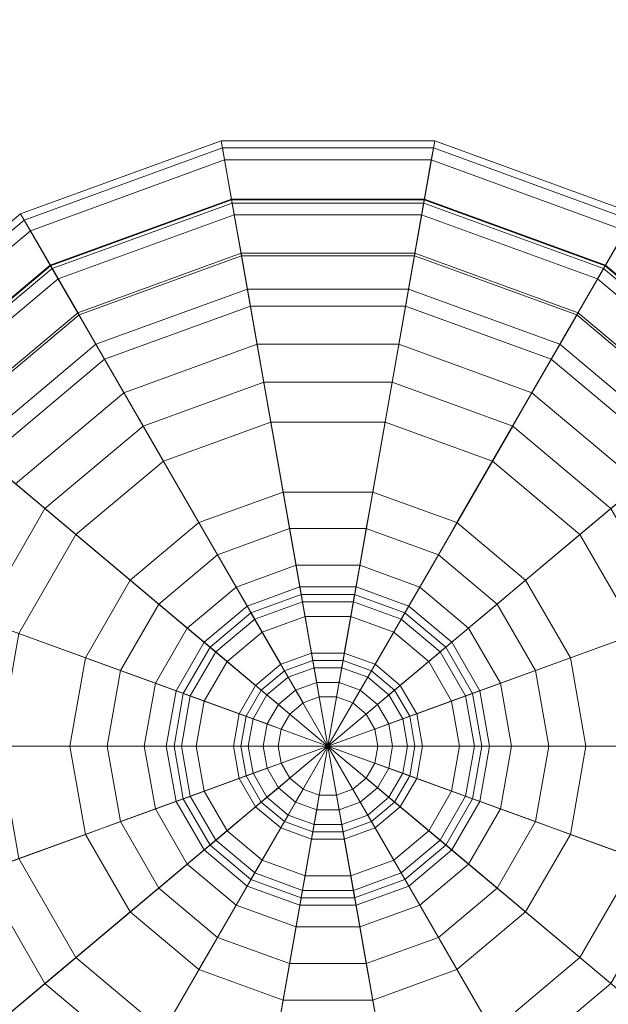
# Model space of a CAD drawing. Units: inches. Extents: x 375 to 1122, y 27 to 1069.
# Tile 110 of 155: x 732.383 to 733.68, y 872.701 to 874.871. Entities that reach past the tile are written whole.
import ezdxf

# ---------------------------------------------------------------- set-up
doc = ezdxf.new("R2010")
doc.units = ezdxf.units.IN
doc.layers.add('A-ANNO-DIMS', color=2, linetype='Continuous', lineweight=18)
doc.layers.add('Furniture', color=30, linetype='Continuous', lineweight=18)
doc.styles.get("Standard").update_dxf_attribs({"font": 'arial.ttf'})
doc.dimstyles.new('ISO-25', dxfattribs={"dimtxt": 12, "dimasz": 2.5, "dimexe": 1.5, "dimexo": 1.5, "dimtad": 1, "dimdec": 1, "dimlunit": 3, "dimtxsty": 'Standard', "dimblk": 'ARCHTICK', "dimcen": 2.5, "dimadec": 0, "dimazin": 0, "dimtfac": 1, "dimtdec": 1, "dimtmove": 0, "dimatfit": 3, "dimfxl": 1.5, "dimfxlon": 1, "dimarcsym": 0})

# ---------------------------------------------------------------- blocks, each defined once
blk = doc.blocks.new('A$C403C54AD')
for points in [[(1.626464, 1.23678, -0.04658), (1.626464, 1.202917, -0.043501), (1.626464, 1.202917, -0.043501), (1.614883, 1.234737, -0.04658)], [(1.638046, 1.234737, -0.04658), (1.626464, 1.202917, -0.043501), (1.626464, 1.202917, -0.043501), (1.626464, 1.23678, -0.04658)], [(1.614883, 1.234737, -0.04658), (1.626464, 1.202917, -0.043501), (1.626464, 1.202917, -0.043501), (1.604698, 1.228857, -0.04658)], [(1.64823, 1.228857, -0.04658), (1.626464, 1.202917, -0.043501), (1.626464, 1.202917, -0.043501), (1.638046, 1.234737, -0.04658)], [(1.626464, 1.217132, -0.040074), (1.626464, 1.233514, -0.043349), (1.616, 1.231669, -0.043349), (1.621603, 1.216274, -0.040074)], [(1.631326, 1.216274, -0.040074), (1.636929, 1.231669, -0.043349), (1.626464, 1.233514, -0.043349), (1.626464, 1.217132, -0.040074)], [(1.621603, 1.216274, -0.040074), (1.616, 1.231669, -0.043349), (1.606797, 1.226356, -0.043349), (1.617327, 1.213806, -0.040074)], [(1.635601, 1.213806, -0.040074), (1.646131, 1.226356, -0.043349), (1.636929, 1.231669, -0.043349), (1.631326, 1.216274, -0.040074)], [(1.604698, 1.228857, -0.04658), (1.626464, 1.202917, -0.043501), (1.626464, 1.202917, -0.043501), (1.597139, 1.219849, -0.04658)], [(1.606797, 1.226356, -0.043349), (1.604698, 1.228857, -0.04658), (1.597139, 1.219849, -0.04658), (1.599967, 1.218216, -0.043349)], [(1.65579, 1.219849, -0.04658), (1.626464, 1.202917, -0.043501), (1.626464, 1.202917, -0.043501), (1.64823, 1.228857, -0.04658)], [(1.606823, 1.226325, 0.116404), (1.604954, 1.228552, 0.10318), (1.597484, 1.219649, 0.10318), (1.600002, 1.218195, 0.116404)], [(1.605388, 1.228035, 0.074938), (1.608836, 1.223925, 0.056929), (1.602714, 1.216629, 0.056929), (1.598069, 1.219312, 0.074938)], [(1.617327, 1.213806, -0.040074), (1.606797, 1.226356, -0.043349), (1.599967, 1.218216, -0.043349), (1.614154, 1.210025, -0.040074)], [(1.610035, 1.222497, 0.12581), (1.606823, 1.226325, 0.116404), (1.600002, 1.218195, 0.116404), (1.604329, 1.215697, 0.12581)], [(1.606937, 1.226189, 0.102963), (1.608743, 1.224037, 0.115599), (1.602589, 1.216702, 0.115599), (1.600155, 1.218107, 0.102963)], [(1.60736, 1.225685, 0.075423), (1.606937, 1.226189, 0.102963), (1.600155, 1.218107, 0.102963), (1.600725, 1.217778, 0.075423)], [(1.620264, 1.219951, 0.048884), (1.618046, 1.226046, 0.058276), (1.610643, 1.221772, 0.058276), (1.614812, 1.216804, 0.048884)], [(1.638116, 1.216804, 0.048884), (1.642285, 1.221772, 0.058276), (1.634882, 1.226046, 0.058276), (1.632664, 1.219951, 0.048884)], [(1.638774, 1.210025, -0.040074), (1.652961, 1.218216, -0.043349), (1.646131, 1.226356, -0.043349), (1.635601, 1.213806, -0.040074)], [(1.610643, 1.221772, 0.058276), (1.60736, 1.225685, 0.075423), (1.600725, 1.217778, 0.075423), (1.605149, 1.215224, 0.058276)], [(1.608743, 1.224037, 0.115599), (1.612014, 1.220139, 0.12581), (1.606995, 1.214158, 0.12581), (1.602589, 1.216702, 0.115599)], [(1.608836, 1.223925, 0.056929), (1.613379, 1.218512, 0.046697), (1.608834, 1.213096, 0.046697), (1.602714, 1.216629, 0.056929)], [(1.650214, 1.216629, 0.056929), (1.644094, 1.213096, 0.046697), (1.63955, 1.218512, 0.046697), (1.644092, 1.223925, 0.056929)], [(1.626464, 1.223275, 0.046697), (1.626464, 1.213036, 0.03933), (1.623003, 1.212426, 0.03933), (1.619501, 1.222047, 0.046697)], [(1.633427, 1.222047, 0.046697), (1.629925, 1.212426, 0.03933), (1.626464, 1.213036, 0.03933), (1.626464, 1.223275, 0.046697)], [(1.612014, 1.220139, 0.12581), (1.610035, 1.222497, 0.12581), (1.604329, 1.215697, 0.12581), (1.606995, 1.214158, 0.12581)], [(1.614812, 1.216804, 0.048884), (1.610643, 1.221772, 0.058276), (1.605149, 1.215224, 0.058276), (1.610766, 1.211981, 0.048884)], [(1.619501, 1.222047, 0.046697), (1.623003, 1.212426, 0.03933), (1.61996, 1.210669, 0.03933), (1.613379, 1.218512, 0.046697)], [(1.63955, 1.218512, 0.046697), (1.632968, 1.210669, 0.03933), (1.629925, 1.212426, 0.03933), (1.633427, 1.222047, 0.046697)], [(1.642163, 1.211981, 0.048884), (1.64778, 1.215224, 0.058276), (1.642285, 1.221772, 0.058276), (1.638116, 1.216804, 0.048884)], [(1.626464, 1.211822, 0.042248), (1.626464, 1.221045, 0.048884), (1.620264, 1.219951, 0.048884), (1.623419, 1.211285, 0.042248)], [(1.62951, 1.211285, 0.042248), (1.632664, 1.219951, 0.048884), (1.626464, 1.221045, 0.048884), (1.626464, 1.211822, 0.042248)], [(1.623419, 1.211285, 0.042248), (1.620264, 1.219951, 0.048884), (1.614812, 1.216804, 0.048884), (1.620741, 1.209738, 0.042248)], [(1.632188, 1.209738, 0.042248), (1.638116, 1.216804, 0.048884), (1.632664, 1.219951, 0.048884), (1.62951, 1.211285, 0.042248)], [(1.597139, 1.219849, -0.04658), (1.626464, 1.202917, -0.043501), (1.626464, 1.202917, -0.043501), (1.593116, 1.208798, -0.04658)], [(1.599967, 1.218216, -0.043349), (1.597139, 1.219849, -0.04658), (1.593116, 1.208798, -0.04658), (1.596333, 1.20823, -0.043349)], [(1.600002, 1.218195, 0.116404), (1.597484, 1.219649, 0.10318), (1.593509, 1.208728, 0.10318), (1.596372, 1.208223, 0.116404)], [(1.597484, 1.219649, 0.10318), (1.598069, 1.219312, 0.074938), (1.594174, 1.208611, 0.074938), (1.593509, 1.208728, 0.10318)], [(1.659812, 1.208798, -0.04658), (1.626464, 1.202917, -0.043501), (1.626464, 1.202917, -0.043501), (1.65579, 1.219849, -0.04658)], [(1.598069, 1.219312, 0.074938), (1.602714, 1.216629, 0.056929), (1.599457, 1.20768, 0.056929), (1.594174, 1.208611, 0.074938)], [(1.613379, 1.218512, 0.046697), (1.61996, 1.210669, 0.03933), (1.617701, 1.207977, 0.03933), (1.608834, 1.213096, 0.046697)], [(1.644094, 1.213096, 0.046697), (1.635227, 1.207977, 0.03933), (1.632968, 1.210669, 0.03933), (1.63955, 1.218512, 0.046697)], [(1.614154, 1.210025, -0.040074), (1.599967, 1.218216, -0.043349), (1.596333, 1.20823, -0.043349), (1.612466, 1.205386, -0.040074)], [(1.604329, 1.215697, 0.12581), (1.600002, 1.218195, 0.116404), (1.596372, 1.208223, 0.116404), (1.601293, 1.207356, 0.12581)], [(1.600155, 1.218107, 0.102963), (1.602589, 1.216702, 0.115599), (1.599314, 1.207705, 0.115599), (1.596547, 1.208193, 0.102963)], [(1.600725, 1.217778, 0.075423), (1.600155, 1.218107, 0.102963), (1.596547, 1.208193, 0.102963), (1.597195, 1.208078, 0.075423)], [(1.605149, 1.215224, 0.058276), (1.600725, 1.217778, 0.075423), (1.597195, 1.208078, 0.075423), (1.602225, 1.207191, 0.058276)], [(1.640462, 1.205386, -0.040074), (1.656596, 1.20823, -0.043349), (1.652961, 1.218216, -0.043349), (1.638774, 1.210025, -0.040074)], [(1.602589, 1.216702, 0.115599), (1.606995, 1.214158, 0.12581), (1.604324, 1.206821, 0.12581), (1.599314, 1.207705, 0.115599)], [(1.620741, 1.209738, 0.042248), (1.614812, 1.216804, 0.048884), (1.610766, 1.211981, 0.048884), (1.618753, 1.207369, 0.042248)], [(1.626464, 1.215084, -0.037209), (1.626464, 1.217132, -0.040074), (1.621603, 1.216274, -0.040074), (1.622303, 1.21435, -0.037209)], [(1.630625, 1.21435, -0.037209), (1.631326, 1.216274, -0.040074), (1.626464, 1.217132, -0.040074), (1.626464, 1.215084, -0.037209)], [(1.634175, 1.207369, 0.042248), (1.642163, 1.211981, 0.048884), (1.638116, 1.216804, 0.048884), (1.632188, 1.209738, 0.042248)], [(1.602714, 1.216629, 0.056929), (1.608834, 1.213096, 0.046697), (1.606416, 1.206452, 0.046697), (1.599457, 1.20768, 0.056929)], [(1.622303, 1.21435, -0.037209), (1.621603, 1.216274, -0.040074), (1.617327, 1.213806, -0.040074), (1.618644, 1.212238, -0.037209)], [(1.634285, 1.212238, -0.037209), (1.635601, 1.213806, -0.040074), (1.631326, 1.216274, -0.040074), (1.630625, 1.21435, -0.037209)], [(1.606995, 1.214158, 0.12581), (1.604329, 1.215697, 0.12581), (1.601293, 1.207356, 0.12581), (1.604324, 1.206821, 0.12581)], [(1.610766, 1.211981, 0.048884), (1.605149, 1.215224, 0.058276), (1.602225, 1.207191, 0.058276), (1.608612, 1.206065, 0.048884)], [(1.626464, 1.210988, -0.035163), (1.626464, 1.215084, -0.037209), (1.622303, 1.21435, -0.037209), (1.623704, 1.210502, -0.035163)], [(1.629225, 1.210502, -0.035163), (1.630625, 1.21435, -0.037209), (1.626464, 1.215084, -0.037209), (1.626464, 1.210988, -0.035163)], [(1.623704, 1.210502, -0.035163), (1.622303, 1.21435, -0.037209), (1.618644, 1.212238, -0.037209), (1.621276, 1.2091, -0.035163)], [(1.631652, 1.2091, -0.035163), (1.634285, 1.212238, -0.037209), (1.630625, 1.21435, -0.037209), (1.629225, 1.210502, -0.035163)], [(1.618644, 1.212238, -0.037209), (1.617327, 1.213806, -0.040074), (1.614154, 1.210025, -0.040074), (1.615928, 1.209001, -0.037209)], [(1.637001, 1.209001, -0.037209), (1.638774, 1.210025, -0.040074), (1.635601, 1.213806, -0.040074), (1.634285, 1.212238, -0.037209)], [(1.608834, 1.213096, 0.046697), (1.617701, 1.207977, 0.03933), (1.616499, 1.204675, 0.03933), (1.606416, 1.206452, 0.046697)], [(1.626464, 1.213036, 0.03933), (1.626464, 1.208122, 0.038511), (1.624684, 1.207808, 0.038511), (1.623003, 1.212426, 0.03933)], [(1.629925, 1.212426, 0.03933), (1.628244, 1.207808, 0.038511), (1.626464, 1.208122, 0.038511), (1.626464, 1.213036, 0.03933)], [(1.646512, 1.206452, 0.046697), (1.636429, 1.204675, 0.03933), (1.635227, 1.207977, 0.03933), (1.644094, 1.213096, 0.046697)], [(1.623003, 1.212426, 0.03933), (1.624684, 1.207808, 0.038511), (1.623119, 1.206904, 0.038511), (1.61996, 1.210669, 0.03933)], [(1.632968, 1.210669, 0.03933), (1.629809, 1.206904, 0.038511), (1.628244, 1.207808, 0.038511), (1.629925, 1.212426, 0.03933)], [(1.618753, 1.207369, 0.042248), (1.610766, 1.211981, 0.048884), (1.608612, 1.206065, 0.048884), (1.617695, 1.204464, 0.042248)], [(1.621276, 1.2091, -0.035163), (1.618644, 1.212238, -0.037209), (1.615928, 1.209001, -0.037209), (1.619474, 1.206953, -0.035163)], [(1.626464, 1.202917, 0.040765), (1.626464, 1.211822, 0.042248), (1.623419, 1.211285, 0.042248), (1.626464, 1.202917, 0.040765)], [(1.626464, 1.202917, 0.040765), (1.62951, 1.211285, 0.042248), (1.626464, 1.211822, 0.042248), (1.626464, 1.202917, 0.040765)], [(1.633454, 1.206953, -0.035163), (1.637001, 1.209001, -0.037209), (1.634285, 1.212238, -0.037209), (1.631652, 1.2091, -0.035163)], [(1.635233, 1.204464, 0.042248), (1.644316, 1.206065, 0.048884), (1.642163, 1.211981, 0.048884), (1.634175, 1.207369, 0.042248)], [(1.626464, 1.202917, 0.040765), (1.623419, 1.211285, 0.042248), (1.620741, 1.209738, 0.042248), (1.626464, 1.202917, 0.040765)], [(1.626464, 1.211398, 0.035646), (1.626464, 1.207302, 0.033599), (1.624964, 1.207038, 0.033599), (1.623564, 1.210887, 0.035646)], [(1.626464, 1.210169, 0.037692), (1.626464, 1.211398, 0.035646), (1.623564, 1.210887, 0.035646), (1.623984, 1.209732, 0.037692)], [(1.629365, 1.210887, 0.035646), (1.627964, 1.207038, 0.033599), (1.626464, 1.207302, 0.033599), (1.626464, 1.211398, 0.035646)], [(1.628944, 1.209732, 0.037692), (1.629365, 1.210887, 0.035646), (1.626464, 1.211398, 0.035646), (1.626464, 1.210169, 0.037692)], [(1.626464, 1.202917, 0.040765), (1.632188, 1.209738, 0.042248), (1.62951, 1.211285, 0.042248), (1.626464, 1.202917, 0.040765)], [(1.623564, 1.210887, 0.035646), (1.624964, 1.207038, 0.033599), (1.623646, 1.206277, 0.033599), (1.621013, 1.209414, 0.035646)], [(1.623984, 1.209732, 0.037692), (1.623564, 1.210887, 0.035646), (1.621013, 1.209414, 0.035646), (1.621803, 1.208473, 0.037692)], [(1.626464, 1.207712, -0.029842), (1.626464, 1.210988, -0.035163), (1.623704, 1.210502, -0.035163), (1.624824, 1.207423, -0.029842)], [(1.628104, 1.207423, -0.029842), (1.629225, 1.210502, -0.035163), (1.626464, 1.210988, -0.035163), (1.626464, 1.207712, -0.029842)], [(1.631915, 1.209414, 0.035646), (1.629283, 1.206277, 0.033599), (1.627964, 1.207038, 0.033599), (1.629365, 1.210887, 0.035646)], [(1.631126, 1.208473, 0.037692), (1.631915, 1.209414, 0.035646), (1.629365, 1.210887, 0.035646), (1.628944, 1.209732, 0.037692)], [(1.61996, 1.210669, 0.03933), (1.623119, 1.206904, 0.038511), (1.621957, 1.205519, 0.038511), (1.617701, 1.207977, 0.03933)], [(1.624824, 1.207423, -0.029842), (1.623704, 1.210502, -0.035163), (1.621276, 1.2091, -0.035163), (1.623382, 1.20659, -0.029842)], [(1.629546, 1.20659, -0.029842), (1.631652, 1.2091, -0.035163), (1.629225, 1.210502, -0.035163), (1.628104, 1.207423, -0.029842)], [(1.635227, 1.207977, 0.03933), (1.630971, 1.205519, 0.038511), (1.629809, 1.206904, 0.038511), (1.632968, 1.210669, 0.03933)], [(1.615928, 1.209001, -0.037209), (1.614154, 1.210025, -0.040074), (1.612466, 1.205386, -0.040074), (1.614482, 1.20503, -0.037209)], [(1.626464, 1.202917, 0.040765), (1.620741, 1.209738, 0.042248), (1.618753, 1.207369, 0.042248), (1.626464, 1.202917, 0.040765)], [(1.624684, 1.207808, 0.038511), (1.623984, 1.209732, 0.037692), (1.621803, 1.208473, 0.037692), (1.623119, 1.206904, 0.038511)], [(1.626464, 1.208122, 0.038511), (1.626464, 1.210169, 0.037692), (1.623984, 1.209732, 0.037692), (1.624684, 1.207808, 0.038511)], [(1.628244, 1.207808, 0.038511), (1.628944, 1.209732, 0.037692), (1.626464, 1.210169, 0.037692), (1.626464, 1.208122, 0.038511)], [(1.626464, 1.202917, 0.040765), (1.634175, 1.207369, 0.042248), (1.632188, 1.209738, 0.042248), (1.626464, 1.202917, 0.040765)], [(1.629809, 1.206904, 0.038511), (1.631126, 1.208473, 0.037692), (1.628944, 1.209732, 0.037692), (1.628244, 1.207808, 0.038511)], [(1.638446, 1.20503, -0.037209), (1.640462, 1.205386, -0.040074), (1.638774, 1.210025, -0.040074), (1.637001, 1.209001, -0.037209)], [(1.621013, 1.209414, 0.035646), (1.623646, 1.206277, 0.033599), (1.622667, 1.20511, 0.033599), (1.61912, 1.207158, 0.035646)], [(1.621803, 1.208473, 0.037692), (1.621013, 1.209414, 0.035646), (1.61912, 1.207158, 0.035646), (1.620184, 1.206543, 0.037692)], [(1.623382, 1.20659, -0.029842), (1.621276, 1.2091, -0.035163), (1.619474, 1.206953, -0.035163), (1.622312, 1.205315, -0.029842)], [(1.633809, 1.207158, 0.035646), (1.630262, 1.20511, 0.033599), (1.629283, 1.206277, 0.033599), (1.631915, 1.209414, 0.035646)], [(1.630616, 1.205315, -0.029842), (1.633454, 1.206953, -0.035163), (1.631652, 1.2091, -0.035163), (1.629546, 1.20659, -0.029842)], [(1.632744, 1.206543, 0.037692), (1.633809, 1.207158, 0.035646), (1.631915, 1.209414, 0.035646), (1.631126, 1.208473, 0.037692)], [(1.593116, 1.208798, -0.04658), (1.626464, 1.202917, -0.043501), (1.626464, 1.202917, -0.043501), (1.593116, 1.197037, -0.04658)], [(1.596333, 1.20823, -0.043349), (1.593116, 1.208798, -0.04658), (1.593116, 1.197037, -0.04658), (1.596333, 1.197604, -0.043349)], [(1.596372, 1.208223, 0.116404), (1.593509, 1.208728, 0.10318), (1.593509, 1.197107, 0.10318), (1.596372, 1.197611, 0.116404)], [(1.593509, 1.208728, 0.10318), (1.594174, 1.208611, 0.074938), (1.594174, 1.197224, 0.074938), (1.593509, 1.197107, 0.10318)], [(1.594174, 1.208611, 0.074938), (1.599457, 1.20768, 0.056929), (1.599457, 1.198155, 0.056929), (1.594174, 1.197224, 0.074938)], [(1.619474, 1.206953, -0.035163), (1.615928, 1.209001, -0.037209), (1.614482, 1.20503, -0.037209), (1.618516, 1.204319, -0.035163)], [(1.659812, 1.197037, -0.04658), (1.626464, 1.202917, -0.043501), (1.626464, 1.202917, -0.043501), (1.659812, 1.208798, -0.04658)], [(1.634413, 1.204319, -0.035163), (1.638446, 1.20503, -0.037209), (1.637001, 1.209001, -0.037209), (1.633454, 1.206953, -0.035163)], [(1.612466, 1.205386, -0.040074), (1.596333, 1.20823, -0.043349), (1.596333, 1.197604, -0.043349), (1.612466, 1.200449, -0.040074)], [(1.601293, 1.207356, 0.12581), (1.596372, 1.208223, 0.116404), (1.596372, 1.197611, 0.116404), (1.601293, 1.198479, 0.12581)], [(1.596547, 1.208193, 0.102963), (1.599314, 1.207705, 0.115599), (1.599314, 1.19813, 0.115599), (1.596547, 1.197642, 0.102963)], [(1.597195, 1.208078, 0.075423), (1.596547, 1.208193, 0.102963), (1.596547, 1.197642, 0.102963), (1.597195, 1.197756, 0.075423)], [(1.602225, 1.207191, 0.058276), (1.597195, 1.208078, 0.075423), (1.597195, 1.197756, 0.075423), (1.602225, 1.198643, 0.058276)], [(1.623119, 1.206904, 0.038511), (1.621803, 1.208473, 0.037692), (1.620184, 1.206543, 0.037692), (1.621957, 1.205519, 0.038511)], [(1.630971, 1.205519, 0.038511), (1.632744, 1.206543, 0.037692), (1.631126, 1.208473, 0.037692), (1.629809, 1.206904, 0.038511)], [(1.640462, 1.200449, -0.040074), (1.656596, 1.197604, -0.043349), (1.656596, 1.20823, -0.043349), (1.640462, 1.205386, -0.040074)], [(1.599314, 1.207705, 0.115599), (1.604324, 1.206821, 0.12581), (1.604324, 1.199014, 0.12581), (1.599314, 1.19813, 0.115599)], [(1.599457, 1.20768, 0.056929), (1.606416, 1.206452, 0.046697), (1.606416, 1.199382, 0.046697), (1.599457, 1.198155, 0.056929)], [(1.617701, 1.207977, 0.03933), (1.621957, 1.205519, 0.038511), (1.621339, 1.203821, 0.038511), (1.616499, 1.204675, 0.03933)], [(1.626464, 1.206483, -0.021247), (1.626464, 1.207712, -0.029842), (1.624824, 1.207423, -0.029842), (1.625245, 1.206268, -0.021247)], [(1.627684, 1.206268, -0.021247), (1.628104, 1.207423, -0.029842), (1.626464, 1.207712, -0.029842), (1.626464, 1.206483, -0.021247)], [(1.636429, 1.204675, 0.03933), (1.631589, 1.203821, 0.038511), (1.630971, 1.205519, 0.038511), (1.635227, 1.207977, 0.03933)], [(1.604324, 1.206821, 0.12581), (1.601293, 1.207356, 0.12581), (1.601293, 1.198479, 0.12581), (1.604324, 1.199014, 0.12581)], [(1.608612, 1.206065, 0.048884), (1.602225, 1.207191, 0.058276), (1.602225, 1.198643, 0.058276), (1.608612, 1.19977, 0.048884)], [(1.626464, 1.202917, 0.040765), (1.618753, 1.207369, 0.042248), (1.617695, 1.204464, 0.042248), (1.626464, 1.202917, 0.040765)], [(1.61912, 1.207158, 0.035646), (1.622667, 1.20511, 0.033599), (1.622146, 1.203679, 0.033599), (1.618112, 1.20439, 0.035646)], [(1.620184, 1.206543, 0.037692), (1.61912, 1.207158, 0.035646), (1.618112, 1.20439, 0.035646), (1.619322, 1.204177, 0.037692)], [(1.622312, 1.205315, -0.029842), (1.619474, 1.206953, -0.035163), (1.618516, 1.204319, -0.035163), (1.621742, 1.20375, -0.029842)], [(1.625245, 1.206268, -0.021247), (1.624824, 1.207423, -0.029842), (1.623382, 1.20659, -0.029842), (1.624172, 1.205649, -0.021247)], [(1.624964, 1.207038, 0.033599), (1.625525, 1.205499, 0.027051), (1.624699, 1.205022, 0.027051), (1.623646, 1.206277, 0.033599)], [(1.626464, 1.207302, 0.033599), (1.626464, 1.205664, 0.027051), (1.625525, 1.205499, 0.027051), (1.624964, 1.207038, 0.033599)], [(1.626464, 1.202917, 0.040765), (1.635233, 1.204464, 0.042248), (1.634175, 1.207369, 0.042248), (1.626464, 1.202917, 0.040765)], [(1.627964, 1.207038, 0.033599), (1.627404, 1.205499, 0.027051), (1.626464, 1.205664, 0.027051), (1.626464, 1.207302, 0.033599)], [(1.629283, 1.206277, 0.033599), (1.62823, 1.205022, 0.027051), (1.627404, 1.205499, 0.027051), (1.627964, 1.207038, 0.033599)], [(1.628756, 1.205649, -0.021247), (1.629546, 1.20659, -0.029842), (1.628104, 1.207423, -0.029842), (1.627684, 1.206268, -0.021247)], [(1.634816, 1.20439, 0.035646), (1.630783, 1.203679, 0.033599), (1.630262, 1.20511, 0.033599), (1.633809, 1.207158, 0.035646)], [(1.631186, 1.20375, -0.029842), (1.634413, 1.204319, -0.035163), (1.633454, 1.206953, -0.035163), (1.630616, 1.205315, -0.029842)], [(1.633606, 1.204177, 0.037692), (1.634816, 1.20439, 0.035646), (1.633809, 1.207158, 0.035646), (1.632744, 1.206543, 0.037692)], [(1.606416, 1.206452, 0.046697), (1.616499, 1.204675, 0.03933), (1.616499, 1.20116, 0.03933), (1.606416, 1.199382, 0.046697)], [(1.621957, 1.205519, 0.038511), (1.620184, 1.206543, 0.037692), (1.619322, 1.204177, 0.037692), (1.621339, 1.203821, 0.038511)], [(1.624172, 1.205649, -0.021247), (1.623382, 1.20659, -0.029842), (1.622312, 1.205315, -0.029842), (1.623376, 1.2047, -0.021247)], [(1.626464, 1.205664, 0.027051), (1.626464, 1.206483, -0.021247), (1.625245, 1.206268, -0.021247), (1.625525, 1.205499, 0.027051)], [(1.627404, 1.205499, 0.027051), (1.627684, 1.206268, -0.021247), (1.626464, 1.206483, -0.021247), (1.626464, 1.205664, 0.027051)], [(1.629552, 1.2047, -0.021247), (1.630616, 1.205315, -0.029842), (1.629546, 1.20659, -0.029842), (1.628756, 1.205649, -0.021247)], [(1.631589, 1.203821, 0.038511), (1.633606, 1.204177, 0.037692), (1.632744, 1.206543, 0.037692), (1.630971, 1.205519, 0.038511)], [(1.646512, 1.199382, 0.046697), (1.636429, 1.20116, 0.03933), (1.636429, 1.204675, 0.03933), (1.646512, 1.206452, 0.046697)], [(1.617695, 1.204464, 0.042248), (1.608612, 1.206065, 0.048884), (1.608612, 1.19977, 0.048884), (1.617695, 1.201371, 0.042248)], [(1.623646, 1.206277, 0.033599), (1.624699, 1.205022, 0.027051), (1.624085, 1.204291, 0.027051), (1.622667, 1.20511, 0.033599)], [(1.625525, 1.205499, 0.027051), (1.625245, 1.206268, -0.021247), (1.624172, 1.205649, -0.021247), (1.624699, 1.205022, 0.027051)], [(1.62823, 1.205022, 0.027051), (1.628756, 1.205649, -0.021247), (1.627684, 1.206268, -0.021247), (1.627404, 1.205499, 0.027051)], [(1.630262, 1.20511, 0.033599), (1.628843, 1.204291, 0.027051), (1.62823, 1.205022, 0.027051), (1.629283, 1.206277, 0.033599)], [(1.635233, 1.201371, 0.042248), (1.644316, 1.19977, 0.048884), (1.644316, 1.206065, 0.048884), (1.635233, 1.204464, 0.042248)], [(1.614482, 1.20503, -0.037209), (1.612466, 1.205386, -0.040074), (1.612466, 1.200449, -0.040074), (1.614482, 1.200805, -0.037209)], [(1.623376, 1.2047, -0.021247), (1.622312, 1.205315, -0.029842), (1.621742, 1.20375, -0.029842), (1.622952, 1.203537, -0.021247)], [(1.624699, 1.205022, 0.027051), (1.624172, 1.205649, -0.021247), (1.623376, 1.2047, -0.021247), (1.624085, 1.204291, 0.027051)], [(1.628843, 1.204291, 0.027051), (1.629552, 1.2047, -0.021247), (1.628756, 1.205649, -0.021247), (1.62823, 1.205022, 0.027051)], [(1.629976, 1.203537, -0.021247), (1.631186, 1.20375, -0.029842), (1.630616, 1.205315, -0.029842), (1.629552, 1.2047, -0.021247)], [(1.638446, 1.200805, -0.037209), (1.640462, 1.200449, -0.040074), (1.640462, 1.205386, -0.040074), (1.638446, 1.20503, -0.037209)], [(1.618516, 1.204319, -0.035163), (1.614482, 1.20503, -0.037209), (1.614482, 1.200805, -0.037209), (1.618516, 1.201516, -0.035163)], [(1.622667, 1.20511, 0.033599), (1.624085, 1.204291, 0.027051), (1.623759, 1.203394, 0.027051), (1.622146, 1.203679, 0.033599)], [(1.630783, 1.203679, 0.033599), (1.629169, 1.203394, 0.027051), (1.628843, 1.204291, 0.027051), (1.630262, 1.20511, 0.033599)], [(1.634413, 1.201516, -0.035163), (1.638446, 1.200805, -0.037209), (1.638446, 1.20503, -0.037209), (1.634413, 1.204319, -0.035163)], [(1.616499, 1.204675, 0.03933), (1.621339, 1.203821, 0.038511), (1.621339, 1.202014, 0.038511), (1.616499, 1.20116, 0.03933)], [(1.626464, 1.202917, 0.040765), (1.617695, 1.204464, 0.042248), (1.617695, 1.201371, 0.042248), (1.626464, 1.202917, 0.040765)], [(1.618112, 1.20439, 0.035646), (1.622146, 1.203679, 0.033599), (1.622146, 1.202156, 0.033599), (1.618112, 1.201445, 0.035646)], [(1.619322, 1.204177, 0.037692), (1.618112, 1.20439, 0.035646), (1.618112, 1.201445, 0.035646), (1.619322, 1.201658, 0.037692)], [(1.621742, 1.20375, -0.029842), (1.618516, 1.204319, -0.035163), (1.618516, 1.201516, -0.035163), (1.621742, 1.202085, -0.029842)], [(1.624085, 1.204291, 0.027051), (1.623376, 1.2047, -0.021247), (1.622952, 1.203537, -0.021247), (1.623759, 1.203394, 0.027051)], [(1.626464, 1.202917, 0.040765), (1.635233, 1.201371, 0.042248), (1.635233, 1.204464, 0.042248), (1.626464, 1.202917, 0.040765)], [(1.629169, 1.203394, 0.027051), (1.629976, 1.203537, -0.021247), (1.629552, 1.2047, -0.021247), (1.628843, 1.204291, 0.027051)], [(1.634816, 1.201445, 0.035646), (1.630783, 1.202156, 0.033599), (1.630783, 1.203679, 0.033599), (1.634816, 1.20439, 0.035646)], [(1.631186, 1.202085, -0.029842), (1.634413, 1.201516, -0.035163), (1.634413, 1.204319, -0.035163), (1.631186, 1.20375, -0.029842)], [(1.636429, 1.20116, 0.03933), (1.631589, 1.202014, 0.038511), (1.631589, 1.203821, 0.038511), (1.636429, 1.204675, 0.03933)], [(1.633606, 1.201658, 0.037692), (1.634816, 1.201445, 0.035646), (1.634816, 1.20439, 0.035646), (1.633606, 1.204177, 0.037692)], [(1.621339, 1.203821, 0.038511), (1.619322, 1.204177, 0.037692), (1.619322, 1.201658, 0.037692), (1.621339, 1.202014, 0.038511)], [(1.622952, 1.203537, -0.021247), (1.621742, 1.20375, -0.029842), (1.621742, 1.202085, -0.029842), (1.622952, 1.202298, -0.021247)], [(1.622146, 1.203679, 0.033599), (1.623759, 1.203394, 0.027051), (1.623759, 1.20244, 0.027051), (1.622146, 1.202156, 0.033599)], [(1.630783, 1.202156, 0.033599), (1.629169, 1.20244, 0.027051), (1.629169, 1.203394, 0.027051), (1.630783, 1.203679, 0.033599)], [(1.629976, 1.202298, -0.021247), (1.631186, 1.202085, -0.029842), (1.631186, 1.20375, -0.029842), (1.629976, 1.203537, -0.021247)], [(1.631589, 1.202014, 0.038511), (1.633606, 1.201658, 0.037692), (1.633606, 1.204177, 0.037692), (1.631589, 1.203821, 0.038511)], [(1.623759, 1.203394, 0.027051), (1.622952, 1.203537, -0.021247), (1.622952, 1.202298, -0.021247), (1.623759, 1.20244, 0.027051)], [(1.629169, 1.20244, 0.027051), (1.629976, 1.202298, -0.021247), (1.629976, 1.203537, -0.021247), (1.629169, 1.203394, 0.027051)], [(1.593116, 1.197037, -0.04658), (1.626464, 1.202917, -0.043501), (1.626464, 1.202917, -0.043501), (1.597139, 1.185986, -0.04658)], [(1.597139, 1.185986, -0.04658), (1.626464, 1.202917, -0.043501), (1.626464, 1.202917, -0.043501), (1.604698, 1.176977, -0.04658)], [(1.604698, 1.176977, -0.04658), (1.626464, 1.202917, -0.043501), (1.626464, 1.202917, -0.043501), (1.614883, 1.171097, -0.04658)], [(1.614883, 1.171097, -0.04658), (1.626464, 1.202917, -0.043501), (1.626464, 1.202917, -0.043501), (1.626464, 1.169055, -0.04658)], [(1.626464, 1.202917, 0.040765), (1.617695, 1.201371, 0.042248), (1.618753, 1.198465, 0.042248), (1.626464, 1.202917, 0.040765)], [(1.626464, 1.202917, 0.040765), (1.618753, 1.198465, 0.042248), (1.620741, 1.196096, 0.042248), (1.626464, 1.202917, 0.040765)], [(1.626464, 1.202917, 0.040765), (1.620741, 1.196096, 0.042248), (1.623419, 1.19455, 0.042248), (1.626464, 1.202917, 0.040765)], [(1.626464, 1.202917, 0.040765), (1.623419, 1.19455, 0.042248), (1.626464, 1.194013, 0.042248), (1.626464, 1.202917, 0.040765)], [(1.626464, 1.202917, 0.040765), (1.62951, 1.19455, 0.042248), (1.632188, 1.196096, 0.042248), (1.626464, 1.202917, 0.040765)], [(1.626464, 1.202917, 0.040765), (1.626464, 1.194013, 0.042248), (1.62951, 1.19455, 0.042248), (1.626464, 1.202917, 0.040765)], [(1.626464, 1.202917, 0.040765), (1.634175, 1.198465, 0.042248), (1.635233, 1.201371, 0.042248), (1.626464, 1.202917, 0.040765)], [(1.626464, 1.202917, 0.040765), (1.632188, 1.196096, 0.042248), (1.634175, 1.198465, 0.042248), (1.626464, 1.202917, 0.040765)], [(1.65579, 1.185986, -0.04658), (1.626464, 1.202917, -0.043501), (1.626464, 1.202917, -0.043501), (1.659812, 1.197037, -0.04658)], [(1.64823, 1.176977, -0.04658), (1.626464, 1.202917, -0.043501), (1.626464, 1.202917, -0.043501), (1.65579, 1.185986, -0.04658)], [(1.638046, 1.171097, -0.04658), (1.626464, 1.202917, -0.043501), (1.626464, 1.202917, -0.043501), (1.64823, 1.176977, -0.04658)], [(1.626464, 1.169055, -0.04658), (1.626464, 1.202917, -0.043501), (1.626464, 1.202917, -0.043501), (1.638046, 1.171097, -0.04658)], [(1.618112, 1.201445, 0.035646), (1.622146, 1.202156, 0.033599), (1.622667, 1.200725, 0.033599), (1.61912, 1.198677, 0.035646)], [(1.621742, 1.202085, -0.029842), (1.618516, 1.201516, -0.035163), (1.619474, 1.198882, -0.035163), (1.622312, 1.20052, -0.029842)], [(1.622952, 1.202298, -0.021247), (1.621742, 1.202085, -0.029842), (1.622312, 1.20052, -0.029842), (1.623376, 1.201134, -0.021247)], [(1.622146, 1.202156, 0.033599), (1.623759, 1.20244, 0.027051), (1.624085, 1.201544, 0.027051), (1.622667, 1.200725, 0.033599)], [(1.623759, 1.20244, 0.027051), (1.622952, 1.202298, -0.021247), (1.623376, 1.201134, -0.021247), (1.624085, 1.201544, 0.027051)], [(1.630262, 1.200725, 0.033599), (1.628843, 1.201544, 0.027051), (1.629169, 1.20244, 0.027051), (1.630783, 1.202156, 0.033599)], [(1.628843, 1.201544, 0.027051), (1.629552, 1.201134, -0.021247), (1.629976, 1.202298, -0.021247), (1.629169, 1.20244, 0.027051)], [(1.629552, 1.201134, -0.021247), (1.630616, 1.20052, -0.029842), (1.631186, 1.202085, -0.029842), (1.629976, 1.202298, -0.021247)], [(1.633809, 1.198677, 0.035646), (1.630262, 1.200725, 0.033599), (1.630783, 1.202156, 0.033599), (1.634816, 1.201445, 0.035646)], [(1.630616, 1.20052, -0.029842), (1.633454, 1.198882, -0.035163), (1.634413, 1.201516, -0.035163), (1.631186, 1.202085, -0.029842)], [(1.618516, 1.201516, -0.035163), (1.614482, 1.200805, -0.037209), (1.615928, 1.196834, -0.037209), (1.619474, 1.198882, -0.035163)], [(1.616499, 1.20116, 0.03933), (1.621339, 1.202014, 0.038511), (1.621957, 1.200315, 0.038511), (1.617701, 1.197858, 0.03933)], [(1.619322, 1.201658, 0.037692), (1.618112, 1.201445, 0.035646), (1.61912, 1.198677, 0.035646), (1.620184, 1.199291, 0.037692)], [(1.621339, 1.202014, 0.038511), (1.619322, 1.201658, 0.037692), (1.620184, 1.199291, 0.037692), (1.621957, 1.200315, 0.038511)], [(1.622667, 1.200725, 0.033599), (1.624085, 1.201544, 0.027051), (1.624699, 1.200813, 0.027051), (1.623646, 1.199558, 0.033599)], [(1.624085, 1.201544, 0.027051), (1.623376, 1.201134, -0.021247), (1.624172, 1.200186, -0.021247), (1.624699, 1.200813, 0.027051)], [(1.629283, 1.199558, 0.033599), (1.62823, 1.200813, 0.027051), (1.628843, 1.201544, 0.027051), (1.630262, 1.200725, 0.033599)], [(1.62823, 1.200813, 0.027051), (1.628756, 1.200186, -0.021247), (1.629552, 1.201134, -0.021247), (1.628843, 1.201544, 0.027051)], [(1.630971, 1.200315, 0.038511), (1.632744, 1.199291, 0.037692), (1.633606, 1.201658, 0.037692), (1.631589, 1.202014, 0.038511)], [(1.635227, 1.197858, 0.03933), (1.630971, 1.200315, 0.038511), (1.631589, 1.202014, 0.038511), (1.636429, 1.20116, 0.03933)], [(1.632744, 1.199291, 0.037692), (1.633809, 1.198677, 0.035646), (1.634816, 1.201445, 0.035646), (1.633606, 1.201658, 0.037692)], [(1.633454, 1.198882, -0.035163), (1.637001, 1.196834, -0.037209), (1.638446, 1.200805, -0.037209), (1.634413, 1.201516, -0.035163)], [(1.606416, 1.199382, 0.046697), (1.616499, 1.20116, 0.03933), (1.617701, 1.197858, 0.03933), (1.608834, 1.192739, 0.046697)], [(1.617695, 1.201371, 0.042248), (1.608612, 1.19977, 0.048884), (1.610766, 1.193854, 0.048884), (1.618753, 1.198465, 0.042248)], [(1.623376, 1.201134, -0.021247), (1.622312, 1.20052, -0.029842), (1.623382, 1.199245, -0.029842), (1.624172, 1.200186, -0.021247)], [(1.628756, 1.200186, -0.021247), (1.629546, 1.199245, -0.029842), (1.630616, 1.20052, -0.029842), (1.629552, 1.201134, -0.021247)], [(1.634175, 1.198465, 0.042248), (1.642163, 1.193854, 0.048884), (1.644316, 1.19977, 0.048884), (1.635233, 1.201371, 0.042248)], [(1.644094, 1.192739, 0.046697), (1.635227, 1.197858, 0.03933), (1.636429, 1.20116, 0.03933), (1.646512, 1.199382, 0.046697)], [(1.612466, 1.200449, -0.040074), (1.596333, 1.197604, -0.043349), (1.599967, 1.187619, -0.043349), (1.614154, 1.19581, -0.040074)], [(1.614482, 1.200805, -0.037209), (1.612466, 1.200449, -0.040074), (1.614154, 1.19581, -0.040074), (1.615928, 1.196834, -0.037209)], [(1.61912, 1.198677, 0.035646), (1.622667, 1.200725, 0.033599), (1.623646, 1.199558, 0.033599), (1.621013, 1.196421, 0.035646)], [(1.622312, 1.20052, -0.029842), (1.619474, 1.198882, -0.035163), (1.621276, 1.196735, -0.035163), (1.623382, 1.199245, -0.029842)], [(1.623646, 1.199558, 0.033599), (1.624699, 1.200813, 0.027051), (1.625525, 1.200336, 0.027051), (1.624964, 1.198797, 0.033599)], [(1.624699, 1.200813, 0.027051), (1.624172, 1.200186, -0.021247), (1.625245, 1.199567, -0.021247), (1.625525, 1.200336, 0.027051)], [(1.627964, 1.198797, 0.033599), (1.627404, 1.200336, 0.027051), (1.62823, 1.200813, 0.027051), (1.629283, 1.199558, 0.033599)], [(1.627404, 1.200336, 0.027051), (1.627684, 1.199567, -0.021247), (1.628756, 1.200186, -0.021247), (1.62823, 1.200813, 0.027051)], [(1.631915, 1.196421, 0.035646), (1.629283, 1.199558, 0.033599), (1.630262, 1.200725, 0.033599), (1.633809, 1.198677, 0.035646)], [(1.629546, 1.199245, -0.029842), (1.631652, 1.196735, -0.035163), (1.633454, 1.198882, -0.035163), (1.630616, 1.20052, -0.029842)], [(1.637001, 1.196834, -0.037209), (1.638774, 1.19581, -0.040074), (1.640462, 1.200449, -0.040074), (1.638446, 1.200805, -0.037209)], [(1.638774, 1.19581, -0.040074), (1.652961, 1.187619, -0.043349), (1.656596, 1.197604, -0.043349), (1.640462, 1.200449, -0.040074)], [(1.617701, 1.197858, 0.03933), (1.621957, 1.200315, 0.038511), (1.623119, 1.198931, 0.038511), (1.61996, 1.195166, 0.03933)], [(1.621957, 1.200315, 0.038511), (1.620184, 1.199291, 0.037692), (1.621803, 1.197362, 0.037692), (1.623119, 1.198931, 0.038511)], [(1.624172, 1.200186, -0.021247), (1.623382, 1.199245, -0.029842), (1.624824, 1.198412, -0.029842), (1.625245, 1.199567, -0.021247)], [(1.624964, 1.198797, 0.033599), (1.625525, 1.200336, 0.027051), (1.626464, 1.200171, 0.027051), (1.626464, 1.198532, 0.033599)], [(1.625525, 1.200336, 0.027051), (1.625245, 1.199567, -0.021247), (1.626464, 1.199352, -0.021247), (1.626464, 1.200171, 0.027051)], [(1.626464, 1.198532, 0.033599), (1.626464, 1.200171, 0.027051), (1.627404, 1.200336, 0.027051), (1.627964, 1.198797, 0.033599)], [(1.626464, 1.200171, 0.027051), (1.626464, 1.199352, -0.021247), (1.627684, 1.199567, -0.021247), (1.627404, 1.200336, 0.027051)], [(1.627684, 1.199567, -0.021247), (1.628104, 1.198412, -0.029842), (1.629546, 1.199245, -0.029842), (1.628756, 1.200186, -0.021247)], [(1.629809, 1.198931, 0.038511), (1.631126, 1.197362, 0.037692), (1.632744, 1.199291, 0.037692), (1.630971, 1.200315, 0.038511)], [(1.632968, 1.195166, 0.03933), (1.629809, 1.198931, 0.038511), (1.630971, 1.200315, 0.038511), (1.635227, 1.197858, 0.03933)], [(1.599457, 1.198155, 0.056929), (1.606416, 1.199382, 0.046697), (1.608834, 1.192739, 0.046697), (1.602714, 1.189206, 0.056929)], [(1.608612, 1.19977, 0.048884), (1.602225, 1.198643, 0.058276), (1.605149, 1.190611, 0.058276), (1.610766, 1.193854, 0.048884)], [(1.621013, 1.196421, 0.035646), (1.623646, 1.199558, 0.033599), (1.624964, 1.198797, 0.033599), (1.623564, 1.194948, 0.035646)], [(1.625245, 1.199567, -0.021247), (1.624824, 1.198412, -0.029842), (1.626464, 1.198123, -0.029842), (1.626464, 1.199352, -0.021247)], [(1.626464, 1.199352, -0.021247), (1.626464, 1.198123, -0.029842), (1.628104, 1.198412, -0.029842), (1.627684, 1.199567, -0.021247)], [(1.629365, 1.194948, 0.035646), (1.627964, 1.198797, 0.033599), (1.629283, 1.199558, 0.033599), (1.631915, 1.196421, 0.035646)], [(1.599314, 1.19813, 0.115599), (1.604324, 1.199014, 0.12581), (1.606995, 1.191677, 0.12581), (1.602589, 1.189133, 0.115599)], [(1.604324, 1.199014, 0.12581), (1.601293, 1.198479, 0.12581), (1.604329, 1.190138, 0.12581), (1.606995, 1.191677, 0.12581)], [(1.619474, 1.198882, -0.035163), (1.615928, 1.196834, -0.037209), (1.618644, 1.193597, -0.037209), (1.621276, 1.196735, -0.035163)], [(1.620184, 1.199291, 0.037692), (1.61912, 1.198677, 0.035646), (1.621013, 1.196421, 0.035646), (1.621803, 1.197362, 0.037692)], [(1.61996, 1.195166, 0.03933), (1.623119, 1.198931, 0.038511), (1.624684, 1.198027, 0.038511), (1.623003, 1.193409, 0.03933)], [(1.623382, 1.199245, -0.029842), (1.621276, 1.196735, -0.035163), (1.623704, 1.195333, -0.035163), (1.624824, 1.198412, -0.029842)], [(1.623119, 1.198931, 0.038511), (1.621803, 1.197362, 0.037692), (1.623984, 1.196103, 0.037692), (1.624684, 1.198027, 0.038511)], [(1.623564, 1.194948, 0.035646), (1.624964, 1.198797, 0.033599), (1.626464, 1.198532, 0.033599), (1.626464, 1.194437, 0.035646)], [(1.626464, 1.194437, 0.035646), (1.626464, 1.198532, 0.033599), (1.627964, 1.198797, 0.033599), (1.629365, 1.194948, 0.035646)], [(1.628104, 1.198412, -0.029842), (1.629225, 1.195333, -0.035163), (1.631652, 1.196735, -0.035163), (1.629546, 1.199245, -0.029842)], [(1.628244, 1.198027, 0.038511), (1.628944, 1.196103, 0.037692), (1.631126, 1.197362, 0.037692), (1.629809, 1.198931, 0.038511)], [(1.629925, 1.193409, 0.03933), (1.628244, 1.198027, 0.038511), (1.629809, 1.198931, 0.038511), (1.632968, 1.195166, 0.03933)], [(1.631126, 1.197362, 0.037692), (1.631915, 1.196421, 0.035646), (1.633809, 1.198677, 0.035646), (1.632744, 1.199291, 0.037692)], [(1.631652, 1.196735, -0.035163), (1.634285, 1.193597, -0.037209), (1.637001, 1.196834, -0.037209), (1.633454, 1.198882, -0.035163)], [(1.601293, 1.198479, 0.12581), (1.596372, 1.197611, 0.116404), (1.600002, 1.187639, 0.116404), (1.604329, 1.190138, 0.12581)], [(1.602225, 1.198643, 0.058276), (1.597195, 1.197756, 0.075423), (1.600725, 1.188057, 0.075423), (1.605149, 1.190611, 0.058276)], [(1.618753, 1.198465, 0.042248), (1.610766, 1.193854, 0.048884), (1.614812, 1.189031, 0.048884), (1.620741, 1.196096, 0.042248)], [(1.624824, 1.198412, -0.029842), (1.623704, 1.195333, -0.035163), (1.626464, 1.194846, -0.035163), (1.626464, 1.198123, -0.029842)], [(1.626464, 1.198123, -0.029842), (1.626464, 1.194846, -0.035163), (1.629225, 1.195333, -0.035163), (1.628104, 1.198412, -0.029842)], [(1.632188, 1.196096, 0.042248), (1.638116, 1.189031, 0.048884), (1.642163, 1.193854, 0.048884), (1.634175, 1.198465, 0.042248)], [(1.594174, 1.197224, 0.074938), (1.599457, 1.198155, 0.056929), (1.602714, 1.189206, 0.056929), (1.598069, 1.186523, 0.074938)], [(1.596547, 1.197642, 0.102963), (1.599314, 1.19813, 0.115599), (1.602589, 1.189133, 0.115599), (1.600155, 1.187728, 0.102963)], [(1.597195, 1.197756, 0.075423), (1.596547, 1.197642, 0.102963), (1.600155, 1.187728, 0.102963), (1.600725, 1.188057, 0.075423)], [(1.608834, 1.192739, 0.046697), (1.617701, 1.197858, 0.03933), (1.61996, 1.195166, 0.03933), (1.613379, 1.187323, 0.046697)], [(1.623003, 1.193409, 0.03933), (1.624684, 1.198027, 0.038511), (1.626464, 1.197713, 0.038511), (1.626464, 1.192799, 0.03933)], [(1.624684, 1.198027, 0.038511), (1.623984, 1.196103, 0.037692), (1.626464, 1.195666, 0.037692), (1.626464, 1.197713, 0.038511)], [(1.626464, 1.197713, 0.038511), (1.626464, 1.195666, 0.037692), (1.628944, 1.196103, 0.037692), (1.628244, 1.198027, 0.038511)], [(1.626464, 1.192799, 0.03933), (1.626464, 1.197713, 0.038511), (1.628244, 1.198027, 0.038511), (1.629925, 1.193409, 0.03933)], [(1.63955, 1.187323, 0.046697), (1.632968, 1.195166, 0.03933), (1.635227, 1.197858, 0.03933), (1.644094, 1.192739, 0.046697)], [(1.596333, 1.197604, -0.043349), (1.593116, 1.197037, -0.04658), (1.597139, 1.185986, -0.04658), (1.599967, 1.187619, -0.043349)], [(1.596372, 1.197611, 0.116404), (1.593509, 1.197107, 0.10318), (1.597484, 1.186186, 0.10318), (1.600002, 1.187639, 0.116404)], [(1.593509, 1.197107, 0.10318), (1.594174, 1.197224, 0.074938), (1.598069, 1.186523, 0.074938), (1.597484, 1.186186, 0.10318)], [(1.621803, 1.197362, 0.037692), (1.621013, 1.196421, 0.035646), (1.623564, 1.194948, 0.035646), (1.623984, 1.196103, 0.037692)], [(1.628944, 1.196103, 0.037692), (1.629365, 1.194948, 0.035646), (1.631915, 1.196421, 0.035646), (1.631126, 1.197362, 0.037692)], [(1.615928, 1.196834, -0.037209), (1.614154, 1.19581, -0.040074), (1.617327, 1.192029, -0.040074), (1.618644, 1.193597, -0.037209)], [(1.621276, 1.196735, -0.035163), (1.618644, 1.193597, -0.037209), (1.622303, 1.191485, -0.037209), (1.623704, 1.195333, -0.035163)], [(1.629225, 1.195333, -0.035163), (1.630625, 1.191485, -0.037209), (1.634285, 1.193597, -0.037209), (1.631652, 1.196735, -0.035163)], [(1.634285, 1.193597, -0.037209), (1.635601, 1.192029, -0.040074), (1.638774, 1.19581, -0.040074), (1.637001, 1.196834, -0.037209)], [(1.620741, 1.196096, 0.042248), (1.614812, 1.189031, 0.048884), (1.620264, 1.185883, 0.048884), (1.623419, 1.19455, 0.042248)], [(1.623984, 1.196103, 0.037692), (1.623564, 1.194948, 0.035646), (1.626464, 1.194437, 0.035646), (1.626464, 1.195666, 0.037692)], [(1.626464, 1.195666, 0.037692), (1.626464, 1.194437, 0.035646), (1.629365, 1.194948, 0.035646), (1.628944, 1.196103, 0.037692)], [(1.62951, 1.19455, 0.042248), (1.632664, 1.185883, 0.048884), (1.638116, 1.189031, 0.048884), (1.632188, 1.196096, 0.042248)], [(1.614154, 1.19581, -0.040074), (1.599967, 1.187619, -0.043349), (1.606797, 1.179479, -0.043349), (1.617327, 1.192029, -0.040074)], [(1.635601, 1.192029, -0.040074), (1.646131, 1.179479, -0.043349), (1.652961, 1.187619, -0.043349), (1.638774, 1.19581, -0.040074)], [(1.613379, 1.187323, 0.046697), (1.61996, 1.195166, 0.03933), (1.623003, 1.193409, 0.03933), (1.619501, 1.183788, 0.046697)], [(1.623704, 1.195333, -0.035163), (1.622303, 1.191485, -0.037209), (1.626464, 1.190751, -0.037209), (1.626464, 1.194846, -0.035163)], [(1.626464, 1.194846, -0.035163), (1.626464, 1.190751, -0.037209), (1.630625, 1.191485, -0.037209), (1.629225, 1.195333, -0.035163)], [(1.633427, 1.183788, 0.046697), (1.629925, 1.193409, 0.03933), (1.632968, 1.195166, 0.03933), (1.63955, 1.187323, 0.046697)], [(1.623419, 1.19455, 0.042248), (1.620264, 1.185883, 0.048884), (1.626464, 1.18479, 0.048884), (1.626464, 1.194013, 0.042248)], [(1.626464, 1.194013, 0.042248), (1.626464, 1.18479, 0.048884), (1.632664, 1.185883, 0.048884), (1.62951, 1.19455, 0.042248)], [(1.610766, 1.193854, 0.048884), (1.605149, 1.190611, 0.058276), (1.610643, 1.184063, 0.058276), (1.614812, 1.189031, 0.048884)], [(1.618644, 1.193597, -0.037209), (1.617327, 1.192029, -0.040074), (1.621603, 1.18956, -0.040074), (1.622303, 1.191485, -0.037209)], [(1.619501, 1.183788, 0.046697), (1.623003, 1.193409, 0.03933), (1.626464, 1.192799, 0.03933), (1.626464, 1.18256, 0.046697)], [(1.626464, 1.18256, 0.046697), (1.626464, 1.192799, 0.03933), (1.629925, 1.193409, 0.03933), (1.633427, 1.183788, 0.046697)], [(1.630625, 1.191485, -0.037209), (1.631326, 1.18956, -0.040074), (1.635601, 1.192029, -0.040074), (1.634285, 1.193597, -0.037209)], [(1.638116, 1.189031, 0.048884), (1.642285, 1.184063, 0.058276), (1.64778, 1.190611, 0.058276), (1.642163, 1.193854, 0.048884)], [(1.602714, 1.189206, 0.056929), (1.608834, 1.192739, 0.046697), (1.613379, 1.187323, 0.046697), (1.608836, 1.18191, 0.056929)], [(1.644092, 1.18191, 0.056929), (1.63955, 1.187323, 0.046697), (1.644094, 1.192739, 0.046697), (1.650214, 1.189206, 0.056929)], [(1.617327, 1.192029, -0.040074), (1.606797, 1.179479, -0.043349), (1.616, 1.174166, -0.043349), (1.621603, 1.18956, -0.040074)], [(1.631326, 1.18956, -0.040074), (1.636929, 1.174166, -0.043349), (1.646131, 1.179479, -0.043349), (1.635601, 1.192029, -0.040074)], [(1.602589, 1.189133, 0.115599), (1.606995, 1.191677, 0.12581), (1.612014, 1.185696, 0.12581), (1.608743, 1.181798, 0.115599)], [(1.606995, 1.191677, 0.12581), (1.604329, 1.190138, 0.12581), (1.610035, 1.183338, 0.12581), (1.612014, 1.185696, 0.12581)], [(1.622303, 1.191485, -0.037209), (1.621603, 1.18956, -0.040074), (1.626464, 1.188703, -0.040074), (1.626464, 1.190751, -0.037209)], [(1.626464, 1.190751, -0.037209), (1.626464, 1.188703, -0.040074), (1.631326, 1.18956, -0.040074), (1.630625, 1.191485, -0.037209)], [(1.604329, 1.190138, 0.12581), (1.600002, 1.187639, 0.116404), (1.606823, 1.17951, 0.116404), (1.610035, 1.183338, 0.12581)], [(1.605149, 1.190611, 0.058276), (1.600725, 1.188057, 0.075423), (1.60736, 1.18015, 0.075423), (1.610643, 1.184063, 0.058276)], [(1.621603, 1.18956, -0.040074), (1.616, 1.174166, -0.043349), (1.626464, 1.172321, -0.043349), (1.626464, 1.188703, -0.040074)], [(1.626464, 1.188703, -0.040074), (1.626464, 1.172321, -0.043349), (1.636929, 1.174166, -0.043349), (1.631326, 1.18956, -0.040074)], [(1.598069, 1.186523, 0.074938), (1.602714, 1.189206, 0.056929), (1.608836, 1.18191, 0.056929), (1.605388, 1.1778, 0.074938)], [(1.600155, 1.187728, 0.102963), (1.602589, 1.189133, 0.115599), (1.608743, 1.181798, 0.115599), (1.606937, 1.179646, 0.102963)], [(1.614812, 1.189031, 0.048884), (1.610643, 1.184063, 0.058276), (1.618046, 1.179789, 0.058276), (1.620264, 1.185883, 0.048884)], [(1.632664, 1.185883, 0.048884), (1.634882, 1.179789, 0.058276), (1.642285, 1.184063, 0.058276), (1.638116, 1.189031, 0.048884)], [(1.600725, 1.188057, 0.075423), (1.600155, 1.187728, 0.102963), (1.606937, 1.179646, 0.102963), (1.60736, 1.18015, 0.075423)], [(1.599967, 1.187619, -0.043349), (1.597139, 1.185986, -0.04658), (1.604698, 1.176977, -0.04658), (1.606797, 1.179479, -0.043349)], [(1.600002, 1.187639, 0.116404), (1.597484, 1.186186, 0.10318), (1.604954, 1.177283, 0.10318), (1.606823, 1.17951, 0.116404)], [(1.608836, 1.18191, 0.056929), (1.613379, 1.187323, 0.046697), (1.619501, 1.183788, 0.046697), (1.617085, 1.177147, 0.056929)], [(1.635844, 1.177147, 0.056929), (1.633427, 1.183788, 0.046697), (1.63955, 1.187323, 0.046697), (1.644092, 1.18191, 0.056929)], [(1.597484, 1.186186, 0.10318), (1.598069, 1.186523, 0.074938), (1.605388, 1.1778, 0.074938), (1.604954, 1.177283, 0.10318)]]:
    blk.add_3dface(points)
blk = doc.blocks.new('_ArchTick')
at = {"color": 0, "linetype": 'ByBlock', "const_width": 0.15}
blk.add_lwpolyline([(-0.5, -0.5), (0.5, 0.5)], dxfattribs=at)
blk = doc.blocks.new('*D88')
at = {"layer": 'A-ANNO-DIMS', "color": 0, "lineweight": -2, "transparency": 16777216}
for p, q in [((731.0073, 1052.5277), (731.0073, 1055.5277)), ((854.0073, 1052.5277), (854.0073, 1055.5277)), ((731.0073, 1054.0277), (854.0073, 1054.0277))]:
    blk.add_line(p, q, dxfattribs=at)
at = {"layer": 'Defpoints', "color": 0, "transparency": 16777216}
for p in [(854.0073, 1054.0277), (731.0073, 502.5277), (854.0073, 502.5277)]:
    blk.add_point(p, dxfattribs=at)
at = {"layer": 'A-ANNO-DIMS', "color": 0, "lineweight": -2, "transparency": 16777216, "xscale": 2.5, "yscale": 2.5, "zscale": 2.5, "rotation": 180}
blk.add_blockref('_ArchTick', (731.0073, 1054.0277), dxfattribs=at)
at = {"layer": 'A-ANNO-DIMS', "color": 0, "lineweight": -2, "transparency": 16777216, "xscale": 2.5, "yscale": 2.5, "zscale": 2.5}
blk.add_blockref('_ArchTick', (854.0073, 1054.0277), dxfattribs=at)
at = {"layer": 'A-ANNO-DIMS', "color": 0, "transparency": 16777216, "insert": (792.5073, 1060.7837), "char_height": 12, "attachment_point": 5}
blk.add_mtext('10\'-3"', dxfattribs=at)
blk = doc.blocks.new('*D91')
at = {"layer": 'A-ANNO-DIMS', "color": 0, "lineweight": -2, "transparency": 16777216}
for p, q in [((728.0073, 1052.5277), (728.0073, 1055.5277)), ((788.0073, 1052.5277), (788.0073, 1055.5277)), ((728.0073, 1054.0277), (788.0073, 1054.0277))]:
    blk.add_line(p, q, dxfattribs=at)
at = {"layer": 'Defpoints', "color": 0, "transparency": 16777216}
for p in [(788.0073, 1054.0277), (728.0073, 774.0277), (788.0073, 774.0277)]:
    blk.add_point(p, dxfattribs=at)
at = {"layer": 'A-ANNO-DIMS', "color": 0, "lineweight": -2, "transparency": 16777216, "xscale": 2.5, "yscale": 2.5, "zscale": 2.5, "rotation": 180}
blk.add_blockref('_ArchTick', (728.0073, 1054.0277), dxfattribs=at)
at = {"layer": 'A-ANNO-DIMS', "color": 0, "lineweight": -2, "transparency": 16777216, "xscale": 2.5, "yscale": 2.5, "zscale": 2.5}
blk.add_blockref('_ArchTick', (788.0073, 1054.0277), dxfattribs=at)
at = {"layer": 'A-ANNO-DIMS', "color": 0, "transparency": 16777216, "insert": (758.0073, 1060.7796), "char_height": 12, "attachment_point": 5}
blk.add_mtext('5\'-0"', dxfattribs=at)

msp = doc.modelspace()

# ---------------------------------------------------------------- block references
at = {"layer": 'Furniture', "xscale": 39.9918517141215, "yscale": 39.9918517141215, "zscale": 39.9918517141215, "rotation": 270}
msp.add_blockref('A$C403C54AD', (684.9549, 938.3156, 0.024), dxfattribs=at)

# ---------------------------------------------------------------- dimensions: what is measured, and where the dimension line sits
at = {"layer": 'A-ANNO-DIMS'}
for base, p1, p2, picture, middle in [((788.0073, 1054.0277), (728.0073, 774.0277), (788.0073, 774.0277), '*D91', (758.0073, 1060.7796)), ((854.0073, 1054.0277), (731.0073, 502.5277), (854.0073, 502.5277), '*D88', (792.5073, 1060.7837))]:
    dim = msp.add_linear_dim(base=base, p1=p1, p2=p2, dimstyle='ISO-25', override={"dimdec": 1, "dimlfac": 1, "dimrnd": 0, "dimzin": 1, "dimdsep": 46, "dimlunit": 4, "dimfrac": 2}, dxfattribs=at)
    dim.commit()
    dim.dimension.update_dxf_attribs({"geometry": picture, "text_midpoint": middle})

doc.saveas('drawing.dxf')
